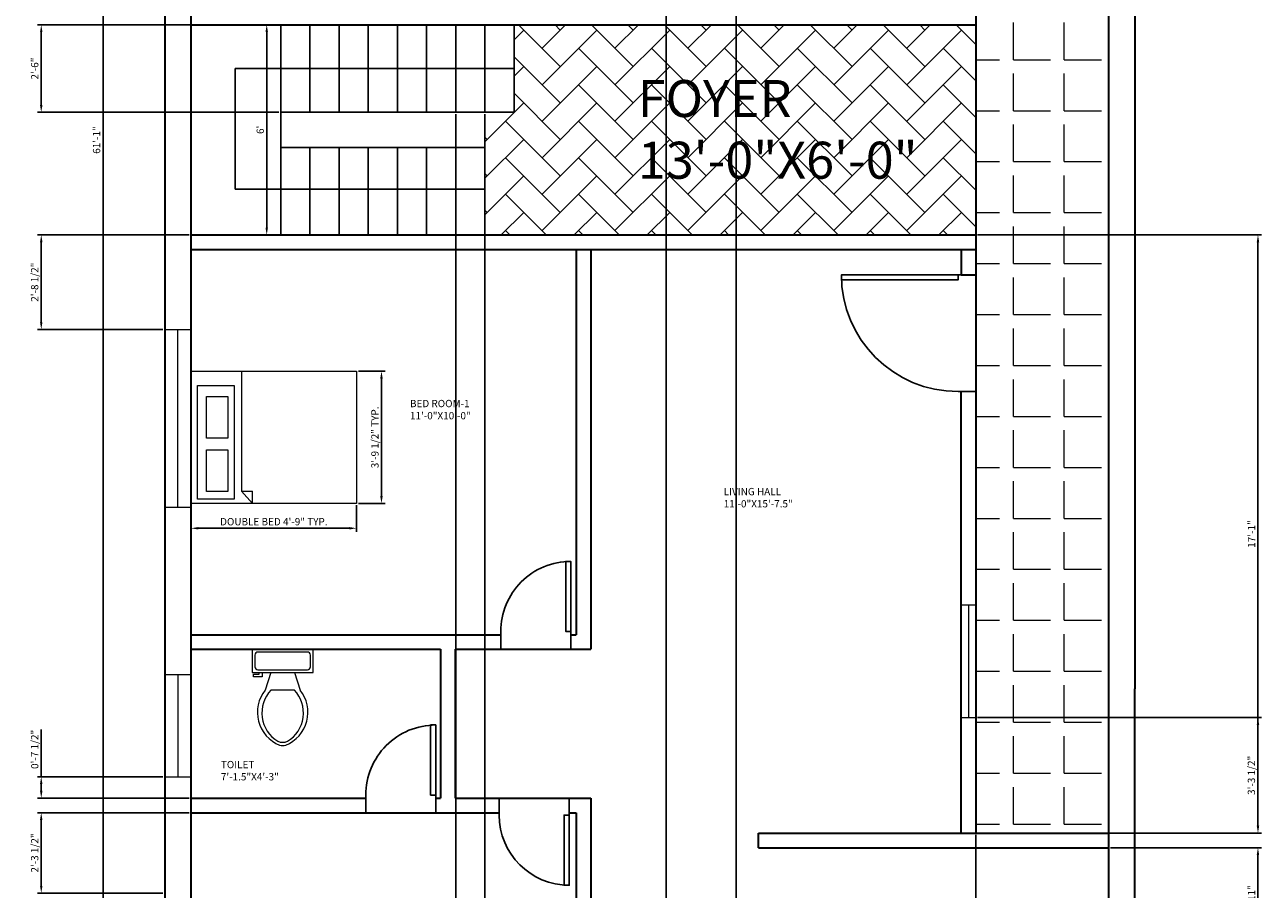
# Model space of a CAD drawing. Units: inches. Extents: x 4673 to 5097, y 7020 to 7947.
# Tile 2 of 3: x 4673 to 5097, y 7225 to 7521. Entities that reach past the tile are written whole.
import ezdxf

# ---------------------------------------------------------------- set-up
doc = ezdxf.new("R2010")
doc.units = ezdxf.units.IN
for name, color, linetype, lineweight in [('A-ANNO-DIMS', 244, 'Continuous', 18), ('A-AREA-IDEN', 7, 'Continuous', 18), ('A-DOOR', 4, 'Continuous', 25), ('A-FLOR-FIXT', 8, 'Continuous', 18), ('A-FLOR-PATT', 9, 'Continuous', 13), ('A-FLOR-STRS', 7, 'Continuous', 25), ('A-FURN', 152, 'Continuous', 18), ('A-GLAZ', 152, 'Continuous', 18), ('A-WALL', 7, 'Continuous', 35)]:
    doc.layers.add(name, color=color, linetype=linetype, lineweight=lineweight)
doc.styles.get("Standard").update_dxf_attribs({"font": 'arial.ttf'})
doc.dimstyles.new('ISO-25', dxfattribs={"dimtxt": 2.5, "dimasz": 2.5, "dimexe": 1.25, "dimexo": 0.625, "dimtad": 1, "dimlunit": 3, "dimtxsty": 'Standard', "dimcen": 2.5, "dimadec": 0, "dimazin": 0, "dimtfac": 1, "dimtmove": 0, "dimatfit": 3, "dimfxl": 1, "dimarcsym": 0})

# ---------------------------------------------------------------- blocks, each defined once
blk = doc.blocks.new('*D1')
at = {"layer": 'A-ANNO-DIMS', "color": 0, "lineweight": -2, "transparency": 16777216}
for p, q in [((4760.01, 7520.86), (4754.6, 7520.86)), ((4755.85, 7518.36), (4755.85, 7451.36)), ((4760.01, 7448.86), (4754.6, 7448.86))]:
    blk.add_line(p, q, dxfattribs=at)
at = {"layer": 'A-ANNO-DIMS', "color": 0, "transparency": 16777216}
for points in [[(4755.43, 7518.36), (4756.27, 7518.36), (4755.85, 7520.86)], [(4755.43, 7451.36), (4756.27, 7451.36), (4755.85, 7448.86)]]:
    blk.add_solid(points, dxfattribs=at)
at = {"layer": 'Defpoints', "color": 0, "transparency": 16777216}
for p in [(4760.64, 7520.86), (4755.85, 7448.86), (4760.64, 7448.86)]:
    blk.add_point(p, dxfattribs=at)
at = {"layer": 'A-ANNO-DIMS', "color": 0, "transparency": 16777216, "insert": (4753.95, 7484.86), "char_height": 2.5, "attachment_point": 5, "rotation": 90}
blk.add_mtext("6'", dxfattribs=at)
blk = doc.blocks.new('*U3')
for p, q in [((0, 0), (0, -6)), ((40, 0), (40, -6))]:
    blk.add_line(p, q)
blk.add_lwpolyline([(0, 0), (0, 40), (1.75, 40), (1.75, 0)], close=True)
blk.add_arc((0, 0), 40, 0, 90)
blk = doc.blocks.new('*U4')
for p, q in [((0, 0), (0, -6)), ((24, 0), (24, -6))]:
    blk.add_line(p, q)
blk.add_lwpolyline([(0, 0), (0, 24), (1.75, 24), (1.75, 0)], close=True)
blk.add_arc((0, 0), 24, 0, 90)
blk = doc.blocks.new('*U5')
for p, q in [((0, 0), (0, 6)), ((24, 0), (24, 6))]:
    blk.add_line(p, q)
blk.add_lwpolyline([(0, 0), (0, -24), (1.75, -24), (1.75, 0)], close=True)
blk.add_arc((0, 0), 24, 270, 0)
blk = doc.blocks.new('*U8')
for p, q in [((9.5, -6), (9.5, -2)), ((-8, -8.5), (-8, -8)), ((-7, -8), (-7, -9.5)), ((-4, -8), (-6, -14)), ((4, -8), (6, -14)), ((-10, -8.5), (-8, -8.5)), ((-10, -9.5), (-10, -8.5)), ((-7, -9.5), (-10, -9.5)), ((4, -14), (-4, -14))]:
    blk.add_line(p, q)
blk.add_lwpolyline([(10.5, -8), (10.5, 0), (-10.5, 0), (-10.5, -8)], close=True)
for points in [[(-9.5, -2), (-9.5, -6)], [(8.5, -1), (-8.5, -1)], [(-8.5, -7), (8.5, -7)]]:
    blk.add_lwpolyline(points)
for centre, radius, start, end in [((-8.62, -1.88), 0.884, 81.8699, 188.1301), ((8.62, -1.88), 0.884, 351.8699, 98.1301), ((-8.62, -6.12), 0.884, 171.8699, 278.1301), ((8.62, -6.12), 0.884, 261.8699, 8.1301), ((3.52, -21.58), 12.17, 141.4691, 247.9714), ((4.2, -21.82), 11.33, 136.3677, 238.9468), ((-3.52, -21.58), 12.17, 292.0284, 38.5307), ((-4.2, -21.82), 11.33, 301.053, 43.6321), ((0, -27.88), 4, 245.7318, 294.2682), ((0, -29), 4, 254.8605, 285.1395)]:
    blk.add_arc(centre, radius, start, end)
blk = doc.blocks.new('*D10')
at = {"layer": 'A-ANNO-DIMS', "color": 0, "lineweight": -2, "transparency": 16777216}
for p, q in [((4720.26, 7847.86), (4698.51, 7847.86)), ((4699.76, 7845.36), (4699.76, 7117.36)), ((4720.26, 7114.86), (4698.51, 7114.86))]:
    blk.add_line(p, q, dxfattribs=at)
at = {"layer": 'A-ANNO-DIMS', "color": 0, "transparency": 16777216}
for points in [[(4699.34, 7845.36), (4700.18, 7845.36), (4699.76, 7847.86)], [(4699.34, 7117.36), (4700.18, 7117.36), (4699.76, 7114.86)]]:
    blk.add_solid(points, dxfattribs=at)
at = {"layer": 'Defpoints', "color": 0, "transparency": 16777216}
for p in [(4720.89, 7847.86), (4699.76, 7114.86), (4720.89, 7114.86)]:
    blk.add_point(p, dxfattribs=at)
at = {"layer": 'A-ANNO-DIMS', "color": 0, "transparency": 16777216, "insert": (4697.86, 7481.36), "char_height": 2.5, "attachment_point": 5, "rotation": 90}
blk.add_mtext('61\'-1"', dxfattribs=at)
blk = doc.blocks.new('BED-DOUBLE')
for p, q in [((17.35, 45.28), (17.35, 4.23)), ((17.35, 4.23), (21.14, 0)), ((17.35, 4.23), (21.14, 4.23)), ((21.14, 0), (21.14, 4.23))]:
    blk.add_line(p, q)
for points in [[(0, 0), (0, 45.28), (56.77, 45.28), (56.77, 0)], [(2.29, 1.5), (2.29, 40.39), (14.79, 40.39), (14.79, 1.5)], [(5.28, 22.37), (5.28, 36.69), (12.64, 36.69), (12.64, 22.37)], [(5.28, 4.03), (5.28, 18.35), (12.64, 18.35), (12.64, 4.03)]]:
    blk.add_lwpolyline(points, close=True)
blk = doc.blocks.new('WIN-61IN')
for p, q in [((9, 60.82), (0, 60.82)), ((0.12, 60.89), (0.12, 0.07)), ((9, 60.82), (4.5, 60.82)), ((4.5, 60.82), (4.5, 0)), ((9.12, 0), (9.12, 60.82)), ((0, 0), (9, 0))]:
    blk.add_line(p, q)
blk = doc.blocks.new('WIN-HALL-38IN')
for p, q in [((5, 38.52), (0, 38.52)), ((0, 38.52), (0, 0)), ((5, 38.52), (2.5, 38.52)), ((2.5, 38.52), (2.5, 0)), ((5, 0), (5, 38.52)), ((0, 0), (5, 0))]:
    blk.add_line(p, q)
blk = doc.blocks.new('WIN-BATH-35IN')
for p, q in [((9, 34.94), (0, 34.94)), ((0, 34.94), (0, 0)), ((9, 34.94), (4.5, 34.94)), ((4.5, 34.94), (4.5, 0)), ((9, 0), (9, 34.94)), ((0, 0), (9, 0))]:
    blk.add_line(p, q)
blk = doc.blocks.new('*D15')
at = {"layer": 'A-ANNO-DIMS', "color": 0, "lineweight": -2, "transparency": 16777216}
for p, q in [((4729.89, 7356.22), (4729.89, 7347.08)), ((4786.66, 7356.22), (4786.66, 7347.08)), ((4732.39, 7348.33), (4784.16, 7348.33))]:
    blk.add_line(p, q, dxfattribs=at)
at = {"layer": 'A-ANNO-DIMS', "color": 0, "transparency": 16777216}
for points in [[(4732.39, 7348.74), (4732.39, 7347.91), (4729.89, 7348.33)], [(4784.16, 7348.74), (4784.16, 7347.91), (4786.66, 7348.33)]]:
    blk.add_solid(points, dxfattribs=at)
at = {"layer": 'Defpoints', "color": 0, "transparency": 16777216}
for p in [(4729.89, 7356.84), (4786.66, 7356.84), (4786.66, 7348.33)]:
    blk.add_point(p, dxfattribs=at)
at = {"layer": 'A-ANNO-DIMS', "color": 0, "transparency": 16777216, "insert": (4758.28, 7350.25), "char_height": 2.5, "attachment_point": 5}
blk.add_mtext('DOUBLE BED 4\'-9" TYP.', dxfattribs=at)
blk = doc.blocks.new('*D16')
at = {"layer": 'A-ANNO-DIMS', "color": 0, "lineweight": -2, "transparency": 16777216}
for p, q in [((4787.29, 7402.12), (4796.43, 7402.12)), ((4795.18, 7359.34), (4795.18, 7399.62)), ((4787.29, 7356.84), (4796.43, 7356.84))]:
    blk.add_line(p, q, dxfattribs=at)
at = {"layer": 'A-ANNO-DIMS', "color": 0, "transparency": 16777216}
for points in [[(4794.76, 7399.62), (4795.6, 7399.62), (4795.18, 7402.12)], [(4794.76, 7359.34), (4795.6, 7359.34), (4795.18, 7356.84)]]:
    blk.add_solid(points, dxfattribs=at)
at = {"layer": 'Defpoints', "color": 0, "transparency": 16777216}
for p in [(4786.66, 7402.12), (4795.18, 7402.12), (4786.66, 7356.84)]:
    blk.add_point(p, dxfattribs=at)
at = {"layer": 'A-ANNO-DIMS', "color": 0, "transparency": 16777216, "insert": (4793.26, 7379.48), "char_height": 2.5, "attachment_point": 5, "rotation": 90}
blk.add_mtext('3\'-9 1/2" TYP.', dxfattribs=at)
blk = doc.blocks.new('*D23')
at = {"layer": 'A-ANNO-DIMS', "color": 0, "lineweight": -2, "transparency": 16777216}
for p, q in [((4998.89, 7243.24), (4998.89, 7020.41)), ((5044.39, 7243.24), (5044.39, 7020.41)), ((5001.39, 7021.66), (5041.89, 7021.66))]:
    blk.add_line(p, q, dxfattribs=at)
at = {"layer": 'A-ANNO-DIMS', "color": 0, "transparency": 16777216}
for points in [[(5001.39, 7022.08), (5001.39, 7021.25), (4998.89, 7021.66)], [(5041.89, 7022.08), (5041.89, 7021.25), (5044.39, 7021.66)]]:
    blk.add_solid(points, dxfattribs=at)
at = {"layer": 'Defpoints', "color": 0, "transparency": 16777216}
for p in [(4998.89, 7243.86), (5044.39, 7243.86), (5044.39, 7021.66)]:
    blk.add_point(p, dxfattribs=at)
at = {"layer": 'A-ANNO-DIMS', "color": 0, "transparency": 16777216, "insert": (5021.64, 7023.58), "char_height": 2.5, "attachment_point": 5}
blk.add_mtext('3\'-9 1/2"', dxfattribs=at)
blk = doc.blocks.new('*D24')
at = {"layer": 'A-ANNO-DIMS', "color": 0, "lineweight": -2, "transparency": 16777216}
for p, q in [((4999.51, 7448.86), (5096.84, 7448.86)), ((5095.59, 7246.36), (5095.59, 7446.36)), ((4999.51, 7243.86), (5096.84, 7243.86))]:
    blk.add_line(p, q, dxfattribs=at)
at = {"layer": 'A-ANNO-DIMS', "color": 0, "transparency": 16777216}
for points in [[(5095.17, 7446.36), (5096.01, 7446.36), (5095.59, 7448.86)], [(5095.17, 7246.36), (5096.01, 7246.36), (5095.59, 7243.86)]]:
    blk.add_solid(points, dxfattribs=at)
at = {"layer": 'Defpoints', "color": 0, "transparency": 16777216}
for p in [(4998.89, 7448.86), (5095.59, 7448.86), (4998.89, 7243.86)]:
    blk.add_point(p, dxfattribs=at)
at = {"layer": 'A-ANNO-DIMS', "color": 0, "transparency": 16777216, "insert": (5093.71, 7346.36), "char_height": 2.5, "attachment_point": 5, "rotation": 90}
blk.add_mtext('17\'-1"', dxfattribs=at)
blk = doc.blocks.new('*D32')
at = {"layer": 'A-ANNO-DIMS', "color": 0, "lineweight": -2, "transparency": 16777216}
for p, q in [((4760.01, 7520.86), (4677.32, 7520.86)), ((4678.57, 7493.36), (4678.57, 7518.36)), ((4760.01, 7490.86), (4677.32, 7490.86))]:
    blk.add_line(p, q, dxfattribs=at)
at = {"layer": 'A-ANNO-DIMS', "color": 0, "transparency": 16777216}
for points in [[(4678.15, 7518.36), (4678.99, 7518.36), (4678.57, 7520.86)], [(4678.15, 7493.36), (4678.99, 7493.36), (4678.57, 7490.86)]]:
    blk.add_solid(points, dxfattribs=at)
at = {"layer": 'Defpoints', "color": 0, "transparency": 16777216}
for p in [(4678.57, 7520.86), (4760.64, 7520.86), (4760.64, 7490.86)]:
    blk.add_point(p, dxfattribs=at)
at = {"layer": 'A-ANNO-DIMS', "color": 0, "transparency": 16777216, "insert": (4676.67, 7505.86), "char_height": 2.5, "attachment_point": 5, "rotation": 90}
blk.add_mtext('2\'-6"', dxfattribs=at)
blk = doc.blocks.new('*D33')
at = {"layer": 'A-ANNO-DIMS', "color": 0, "lineweight": -2, "transparency": 16777216}
for p, q in [((4820.64, 7490.24), (4820.64, 7020.41)), ((4830.64, 7490.24), (4830.64, 7020.41)), ((4823.14, 7021.66), (4828.14, 7021.66))]:
    blk.add_line(p, q, dxfattribs=at)
at = {"layer": 'A-ANNO-DIMS', "color": 0, "transparency": 16777216}
for points in [[(4823.14, 7022.08), (4823.14, 7021.25), (4820.64, 7021.66)], [(4828.14, 7022.08), (4828.14, 7021.25), (4830.64, 7021.66)]]:
    blk.add_solid(points, dxfattribs=at)
at = {"layer": 'Defpoints', "color": 0, "transparency": 16777216}
for p in [(4820.64, 7490.86), (4830.64, 7490.86), (4830.64, 7021.66)]:
    blk.add_point(p, dxfattribs=at)
at = {"layer": 'A-ANNO-DIMS', "color": 0, "transparency": 16777216, "insert": (4825.64, 7023.56), "char_height": 2.5, "attachment_point": 5}
blk.add_mtext('0\'-10"', dxfattribs=at)
blk = doc.blocks.new('*D35')
at = {"layer": 'A-ANNO-DIMS', "color": 0, "lineweight": -2, "transparency": 16777216}
for p, q in [((4892.8, 7756.68), (4892.8, 7020.41)), ((4916.8, 7756.68), (4916.8, 7020.41)), ((4895.3, 7021.66), (4914.3, 7021.66))]:
    blk.add_line(p, q, dxfattribs=at)
at = {"layer": 'A-ANNO-DIMS', "color": 0, "transparency": 16777216}
for points in [[(4895.3, 7022.08), (4895.3, 7021.25), (4892.8, 7021.66)], [(4914.3, 7022.08), (4914.3, 7021.25), (4916.8, 7021.66)]]:
    blk.add_solid(points, dxfattribs=at)
at = {"layer": 'Defpoints', "color": 0, "transparency": 16777216}
for p in [(4892.8, 7757.31), (4916.8, 7757.31), (4916.8, 7021.66)]:
    blk.add_point(p, dxfattribs=at)
at = {"layer": 'A-ANNO-DIMS', "color": 0, "transparency": 16777216, "insert": (4904.8, 7023.56), "char_height": 2.5, "attachment_point": 5}
blk.add_mtext('2\'-0"', dxfattribs=at)
blk = doc.blocks.new('*D37')
at = {"layer": 'A-ANNO-DIMS', "color": 0, "lineweight": -2, "transparency": 16777216}
for p, q in [((4729.26, 7250.86), (4677.32, 7250.86)), ((4678.57, 7225.75), (4678.57, 7248.36)), ((4720.26, 7223.25), (4677.32, 7223.25))]:
    blk.add_line(p, q, dxfattribs=at)
at = {"layer": 'A-ANNO-DIMS', "color": 0, "transparency": 16777216}
for points in [[(4678.15, 7248.36), (4678.99, 7248.36), (4678.57, 7250.86)], [(4678.15, 7225.75), (4678.99, 7225.75), (4678.57, 7223.25)]]:
    blk.add_solid(points, dxfattribs=at)
at = {"layer": 'Defpoints', "color": 0, "transparency": 16777216}
for p in [(4678.57, 7250.86), (4729.89, 7250.86), (4720.89, 7223.25)]:
    blk.add_point(p, dxfattribs=at)
at = {"layer": 'A-ANNO-DIMS', "color": 0, "transparency": 16777216, "insert": (4676.65, 7237.05), "char_height": 2.5, "attachment_point": 5, "rotation": 90}
blk.add_mtext('2\'-3 1/2"', dxfattribs=at)
blk = doc.blocks.new('*D38')
at = {"layer": 'A-ANNO-DIMS', "color": 0, "lineweight": -2, "transparency": 16777216}
for p, q in [((4678.57, 7263.19), (4678.57, 7279.42)), ((4720.26, 7263.19), (4677.32, 7263.19)), ((4678.57, 7258.36), (4678.57, 7260.69)), ((4729.26, 7255.86), (4677.32, 7255.86))]:
    blk.add_line(p, q, dxfattribs=at)
at = {"layer": 'A-ANNO-DIMS', "color": 0, "transparency": 16777216}
for points in [[(4678.15, 7260.69), (4678.99, 7260.69), (4678.57, 7263.19)], [(4678.15, 7258.36), (4678.99, 7258.36), (4678.57, 7255.86)]]:
    blk.add_solid(points, dxfattribs=at)
at = {"layer": 'Defpoints', "color": 0, "transparency": 16777216}
for p in [(4678.57, 7263.19), (4720.89, 7263.19), (4729.89, 7255.86)]:
    blk.add_point(p, dxfattribs=at)
at = {"layer": 'A-ANNO-DIMS', "color": 0, "transparency": 16777216, "insert": (4676.65, 7272.56), "char_height": 2.5, "attachment_point": 5, "rotation": 90}
blk.add_mtext('0\'-7 1/2"', dxfattribs=at)
blk = doc.blocks.new('*D39')
at = {"layer": 'A-ANNO-DIMS', "color": 0, "lineweight": -2, "transparency": 16777216}
for p, q in [((4729.26, 7448.86), (4677.32, 7448.86)), ((4678.57, 7418.94), (4678.57, 7446.36)), ((4720.26, 7416.44), (4677.32, 7416.44))]:
    blk.add_line(p, q, dxfattribs=at)
at = {"layer": 'A-ANNO-DIMS', "color": 0, "transparency": 16777216}
for points in [[(4678.15, 7446.36), (4678.99, 7446.36), (4678.57, 7448.86)], [(4678.15, 7418.94), (4678.99, 7418.94), (4678.57, 7416.44)]]:
    blk.add_solid(points, dxfattribs=at)
at = {"layer": 'Defpoints', "color": 0, "transparency": 16777216}
for p in [(4678.57, 7448.86), (4729.89, 7448.86), (4720.89, 7416.44)]:
    blk.add_point(p, dxfattribs=at)
at = {"layer": 'A-ANNO-DIMS', "color": 0, "transparency": 16777216, "insert": (4676.65, 7432.65), "char_height": 2.5, "attachment_point": 5, "rotation": 90}
blk.add_mtext('2\'-8 1/2"', dxfattribs=at)
blk = doc.blocks.new('*D44')
at = {"layer": 'A-ANNO-DIMS', "color": 0, "lineweight": -2, "transparency": 16777216}
for p, q in [((5045.01, 7238.86), (5096.84, 7238.86)), ((5095.59, 7206.13), (5095.59, 7236.36)), ((5053.89, 7203.63), (5096.84, 7203.63))]:
    blk.add_line(p, q, dxfattribs=at)
at = {"layer": 'A-ANNO-DIMS', "color": 0, "transparency": 16777216}
for points in [[(5095.17, 7236.36), (5096.01, 7236.36), (5095.59, 7238.86)], [(5095.17, 7206.13), (5096.01, 7206.13), (5095.59, 7203.63)]]:
    blk.add_solid(points, dxfattribs=at)
at = {"layer": 'Defpoints', "color": 0, "transparency": 16777216}
for p in [(5044.39, 7238.86), (5095.59, 7238.86), (5053.27, 7203.63)]:
    blk.add_point(p, dxfattribs=at)
at = {"layer": 'A-ANNO-DIMS', "color": 0, "transparency": 16777216, "insert": (5093.71, 7221.25), "char_height": 2.5, "attachment_point": 5, "rotation": 90}
blk.add_mtext('2\'-11"', dxfattribs=at)
blk = doc.blocks.new('*D45')
at = {"layer": 'A-ANNO-DIMS', "color": 0, "lineweight": -2, "transparency": 16777216}
for p, q in [((4999.5, 7283.45), (5096.84, 7283.45)), ((5095.59, 7246.36), (5095.59, 7280.95)), ((4999.51, 7243.86), (5096.84, 7243.86))]:
    blk.add_line(p, q, dxfattribs=at)
at = {"layer": 'A-ANNO-DIMS', "color": 0, "transparency": 16777216}
for points in [[(5095.17, 7280.95), (5096.01, 7280.95), (5095.59, 7283.45)], [(5095.17, 7246.36), (5096.01, 7246.36), (5095.59, 7243.86)]]:
    blk.add_solid(points, dxfattribs=at)
at = {"layer": 'Defpoints', "color": 0, "transparency": 16777216}
for p in [(4998.87, 7283.45), (5095.59, 7283.45), (4998.89, 7243.86)]:
    blk.add_point(p, dxfattribs=at)
at = {"layer": 'A-ANNO-DIMS', "color": 0, "transparency": 16777216, "insert": (5093.67, 7263.66), "char_height": 2.5, "attachment_point": 5, "rotation": 90}
blk.add_mtext('3\'-3 1/2"', dxfattribs=at)

msp = doc.modelspace()

# ---------------------------------------------------------------- hatches: boundary and pattern name
at = {"layer": 'A-FLOR-PATT'}
h = msp.add_hatch(dxfattribs=at)
h.set_pattern_fill('ANGLE', color=256, scale=2.5)
h.set_pattern_definition([(0, (0, 0), (0, 17.4625), [12.7, -4.7625]), (90, (0, 0), (-17.4625, 1e-15), [12.7, -4.7625])])
h.paths.add_polyline_path([(5044.389, 7713.863), (4998.889, 7713.863), (4998.889, 7243.863), (5044.389, 7243.863)])
h = msp.add_hatch(dxfattribs=at)
h.set_pattern_fill('AR-HBONE', color=256, scale=0.087)
h.paths.add_polyline_path([(4998.889, 7520.863), (4840.639, 7520.863), (4840.639, 7490.863), (4830.639, 7490.863), (4830.639, 7478.863), (4830.639, 7448.863), (4998.889, 7448.863)])

# ---------------------------------------------------------------- linework, layer by layer
at = {"layer": 'A-FLOR-STRS'}
for p, q in [((4760.639, 7520.863), (4760.639, 7448.863)), ((4760.639, 7520.863), (4760.639, 7484.863)), ((4760.639, 7520.863), (4760.639, 7496.863)), ((4760.639, 7520.863), (4760.639, 7490.863)), ((4770.639, 7520.863), (4770.639, 7490.863)), ((4780.639, 7520.863), (4780.639, 7490.863)), ((4790.639, 7520.863), (4790.639, 7490.863)), ((4800.639, 7520.863), (4800.639, 7490.863)), ((4810.639, 7520.863), (4810.639, 7490.863)), ((4820.639, 7520.863), (4820.639, 7490.863)), ((4830.639, 7520.863), (4830.639, 7490.863)), ((4840.639, 7520.863), (4840.639, 7490.863)), ((4840.639, 7505.863), (4745.075, 7505.863)), ((4745.075, 7505.863), (4745.075, 7464.475)), ((4760.639, 7490.863), (4840.639, 7490.863)), ((4760.639, 7448.863), (4760.639, 7484.863)), ((4760.639, 7448.863), (4760.639, 7484.863)), ((4760.639, 7448.863), (4760.639, 7478.863)), ((4760.639, 7478.863), (4830.639, 7478.863)), ((4770.639, 7448.863), (4770.639, 7478.863)), ((4780.639, 7448.863), (4780.639, 7478.863)), ((4790.639, 7448.863), (4790.639, 7478.863)), ((4800.639, 7448.863), (4800.639, 7478.863)), ((4810.639, 7448.863), (4810.639, 7478.863)), ((4820.639, 7448.863), (4820.639, 7478.863)), ((4830.639, 7448.863), (4830.639, 7478.863)), ((4760.639, 7448.863), (4760.639, 7472.863)), ((4745.075, 7464.475), (4830.639, 7464.475))]:
    msp.add_line(p, q, dxfattribs=at)
at = {"layer": 'A-WALL'}
for p, q in [((4720.889, 7847.863), (4720.889, 7114.863)), ((5053.389, 7847.863), (5053.389, 7293.326)), ((4998.889, 7713.863), (4998.889, 7243.863)), ((5044.389, 7713.863), (5044.389, 7238.863)), ((4729.889, 7525.863), (4729.889, 7443.863)), ((4729.889, 7520.863), (4861.889, 7520.863)), ((4729.889, 7520.863), (4998.889, 7520.863)), ((4729.889, 7448.863), (4998.889, 7448.863)), ((4729.889, 7448.863), (4729.889, 7311.863)), ((4729.889, 7443.863), (4998.889, 7443.863)), ((4861.889, 7443.863), (4861.889, 7311.863)), ((4866.889, 7443.863), (4866.889, 7306.863)), ((4993.913, 7443.863), (4993.913, 7435.161)), ((4993.913, 7435.161), (4998.889, 7435.161)), ((4993.889, 7243.845), (4993.889, 7395.162)), ((4729.889, 7311.863), (4836.063, 7311.863)), ((4729.889, 7311.863), (4729.889, 7250.863)), ((4860.063, 7311.863), (4861.889, 7311.863)), ((4729.889, 7306.863), (4815.389, 7306.863)), ((4815.389, 7306.863), (4815.389, 7255.863)), ((4820.389, 7306.863), (4820.389, 7255.863)), ((4820.389, 7306.863), (4866.889, 7306.863)), ((5053.389, 7114.863), (5053.389, 7293.326)), ((4729.889, 7255.863), (4789.79, 7255.863)), ((4813.79, 7255.863), (4815.389, 7255.863)), ((4820.389, 7255.863), (4866.889, 7255.863)), ((4866.889, 7255.863), (4866.889, 7205.363)), ((4729.889, 7250.863), (4835.526, 7250.863)), ((4729.889, 7250.863), (4729.889, 7123.863)), ((4859.526, 7250.863), (4861.889, 7250.863)), ((4861.889, 7250.863), (4861.889, 7123.863)), ((4924.389, 7238.863), (4924.389, 7243.863)), ((4924.389, 7243.863), (5044.389, 7243.863)), ((4924.389, 7238.863), (5044.389, 7238.863)), ((5044.389, 7238.863), (5044.389, 7123.863))]:
    msp.add_line(p, q, dxfattribs=at)

# ---------------------------------------------------------------- block references
at = {"layer": 'A-DOOR', "xscale": -1, "rotation": 90}
msp.add_blockref('*U3', (4992.804, 7435.162), dxfattribs=at)
at = {"layer": 'A-DOOR', "rotation": 180}
for name, p in [('*U5', (4860.063, 7312.974)), ('*U5', (4813.79, 7256.911)), ('*U4', (4859.526, 7250.015))]:
    msp.add_blockref(name, p, dxfattribs=at)
at = {"layer": 'A-FLOR-FIXT'}
msp.add_blockref('*U8', (4761.316, 7306.863), dxfattribs=at)
at = {"layer": 'A-FURN'}
msp.add_blockref('BED-DOUBLE', (4729.889, 7356.844), dxfattribs=at)
at = {"layer": 'A-GLAZ'}
for name, p in [('WIN-61IN', (4720.769, 7355.554)), ('WIN-HALL-38IN', (4993.875, 7283.447)), ('WIN-BATH-35IN', (4720.889, 7263.195))]:
    msp.add_blockref(name, p, dxfattribs=at)

# ---------------------------------------------------------------- texts
at = {"layer": 'A-AREA-IDEN', "attachment_point": 1}
for s, width, gutter_width, insert, char_height in [('FOYER\\P13\'-0"X6\'-0"', 410.56001, 63.379, (4883.02, 7501.92), 12.67584), ('BED ROOM-1\\P11\'-0"X10\'-0"', 39.54114, 12.5, (4804.949, 7392.317), 2.5), ('LIVING HALL\\P11\'-0"X15\'-7.5"', 55.14415, 12.5, (4912.483, 7362.141), 2.5), ('TOILET\\P7\'-1.5"X4\'-3"', 44.17753, 12.5, (4740.138, 7268.594), 2.5)]:
    msp.add_mtext_dynamic_manual_height_columns(s, width=width, gutter_width=gutter_width, heights=[0], dxfattribs=dict(at, insert=insert, char_height=char_height))

# ---------------------------------------------------------------- dimensions: what is measured, and where the dimension line sits
at = {"layer": 'A-ANNO-DIMS'}
for base, p1, p2, override, picture, middle in [((4699.76, 7114.863), (4720.889, 7847.863), (4720.889, 7114.863), {"dimclrd": 0, "dimclre": 0, "dimclrt": 0}, '*D10', (4697.858, 7481.363)), ((4678.569, 7520.863), (4760.639, 7490.863), (4760.639, 7520.863), {"dimdec": 1, "dimlfac": 1, "dimrnd": 0, "dimzin": 1, "dimdsep": 46, "dimlunit": 4, "dimfrac": 2}, '*D32', (4676.668, 7505.863)), ((4755.849, 7448.863), (4760.639, 7520.863), (4760.639, 7448.863), {"dimclrd": 0, "dimclre": 0, "dimclrt": 0}, '*D1', (4753.948, 7484.863)), ((4678.569, 7448.863), (4720.889, 7416.44), (4729.889, 7448.863), {"dimdec": 1, "dimlfac": 1, "dimrnd": 0, "dimzin": 1, "dimdsep": 46, "dimlunit": 4, "dimfrac": 2}, '*D39', (4676.652, 7432.652)), ((5095.589, 7448.863), (4998.889, 7243.863), (4998.889, 7448.863), {"dimdec": 1, "dimlfac": 1, "dimrnd": 0, "dimzin": 1, "dimdsep": 46, "dimlunit": 4, "dimfrac": 2}, '*D24', (5093.708, 7346.363)), ((5095.589, 7283.448), (4998.889, 7243.863), (4998.875, 7283.448), {"dimdec": 1, "dimlfac": 1, "dimrnd": 0, "dimzin": 1, "dimdsep": 46, "dimlunit": 4, "dimfrac": 2}, '*D45', (5093.67, 7263.655)), ((4678.569, 7263.195), (4729.889, 7255.863), (4720.889, 7263.195), {"dimdec": 1, "dimlfac": 1, "dimrnd": 0, "dimzin": 1, "dimdsep": 46, "dimlunit": 4, "dimfrac": 2}, '*D38', (4676.652, 7272.555)), ((4678.569, 7250.863), (4720.889, 7223.246), (4729.889, 7250.863), {"dimdec": 1, "dimlfac": 1, "dimrnd": 0, "dimzin": 1, "dimdsep": 46, "dimlunit": 4, "dimfrac": 2}, '*D37', (4676.651, 7237.054)), ((5095.589, 7238.863), (5053.269, 7203.63), (5044.389, 7238.863), {"dimdec": 1, "dimlfac": 1, "dimrnd": 0, "dimzin": 1, "dimdsep": 46, "dimlunit": 4, "dimfrac": 2}, '*D44', (5093.708, 7221.246))]:
    dim = msp.add_linear_dim(base=base, p1=p1, p2=p2, angle=90, dimstyle='ISO-25', override=override, dxfattribs=at)
    dim.commit()
    dim.dimension.update_dxf_attribs({"geometry": picture, "text_midpoint": middle})
for base, p1, p2, picture, middle in [((4916.804, 7021.663), (4892.804, 7757.308), (4916.804, 7757.308), '*D35', (4904.804, 7023.564)), ((4830.639, 7021.663), (4820.639, 7490.863), (4830.639, 7490.863), '*D33', (4825.639, 7023.564)), ((5044.389, 7021.663), (4998.889, 7243.863), (5044.389, 7243.863), '*D23', (5021.639, 7023.581))]:
    dim = msp.add_linear_dim(base=base, p1=p1, p2=p2, dimstyle='ISO-25', override={"dimdec": 1, "dimlfac": 1, "dimrnd": 0, "dimzin": 1, "dimdsep": 46, "dimlunit": 4, "dimfrac": 2}, dxfattribs=at)
    dim.commit()
    dim.dimension.update_dxf_attribs({"geometry": picture, "text_midpoint": middle})
dim = msp.add_linear_dim(base=(4795.178, 7402.124), p1=(4786.662, 7356.844), p2=(4786.662, 7402.124), angle=90, text='<> TYP.', dimstyle='ISO-25', override={"dimdec": 1, "dimlfac": 1, "dimrnd": 0, "dimzin": 1, "dimdsep": 46, "dimlunit": 4, "dimfrac": 2}, dxfattribs=at)
dim.commit()
dim.dimension.update_dxf_attribs({"geometry": '*D16', "text_midpoint": (4793.26, 7379.484)})
dim = msp.add_linear_dim(base=(4786.662, 7348.328), p1=(4729.889, 7356.844), p2=(4786.662, 7356.844), text='DOUBLE BED <> TYP.', dimstyle='ISO-25', override={"dimdec": 1, "dimlfac": 1, "dimrnd": 0, "dimzin": 1, "dimdsep": 46, "dimlunit": 4, "dimfrac": 2}, dxfattribs=at)
dim.commit()
dim.dimension.update_dxf_attribs({"geometry": '*D15', "text_midpoint": (4758.275, 7350.246)})

doc.saveas('drawing.dxf')
